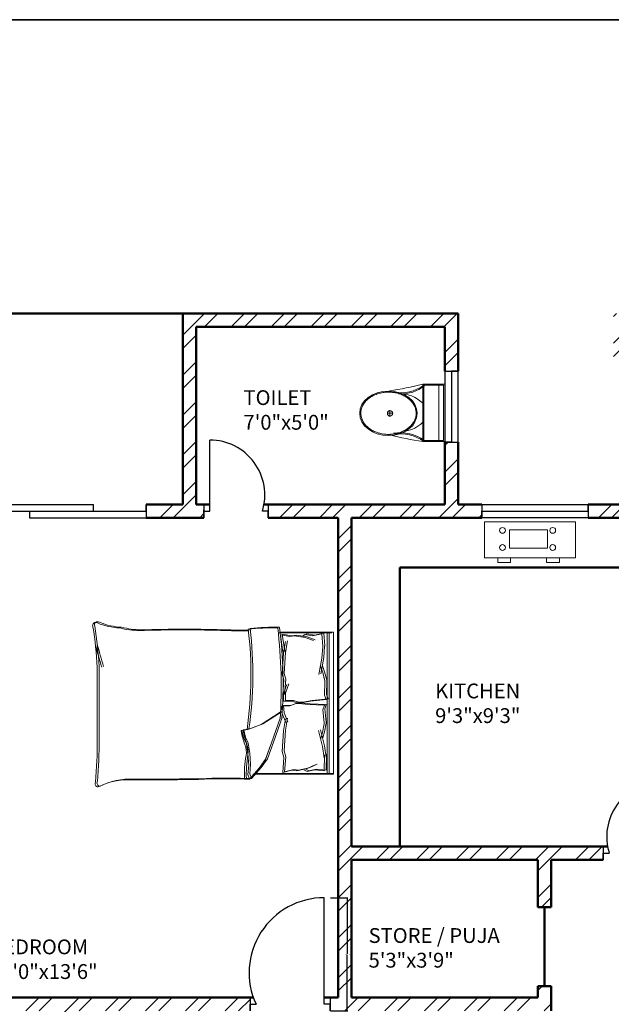
# Model space of a CAD drawing. Units: inches. Extents: x 963 to 2075, y 289 to 2657.
# Tile 80 of 98: x 1149 to 1349, y 2325 to 2657. Entities that reach past the tile are written whole.
import ezdxf

# ---------------------------------------------------------------- set-up
doc = ezdxf.new("R2010")
doc.units = ezdxf.units.IN
for name, color, linetype, lineweight in [('A-ANNO-DIMS', 2, 'Continuous', 18), ('A-ANNO-TTLB', 7, 'Continuous', 35), ('A-AREA-IDEN', 7, 'Continuous', 18), ('A-DOOR', 4, 'Continuous', 25), ('A-FLOR-FIXT', 9, 'Continuous', 18), ('A-FURN', 8, 'Continuous', 18), ('A-GLAZ', 3, 'Continuous', 25), ('A-WALL', 7, 'Continuous', 50), ('A-WALL-PATT', 8, 'Continuous', 13)]:
    doc.layers.add(name, color=color, linetype=linetype, lineweight=lineweight)
doc.styles.get("Standard").update_dxf_attribs({"font": 'arial.ttf'})
doc.dimstyles.get("Standard").update_dxf_attribs({"dimtxt": 0.18, "dimasz": 0.18, "dimexe": 0.18, "dimexo": 0.0625, "dimgap": 0.09, "dimtad": 0, "dimtih": 1, "dimtoh": 1, "dimdec": 4, "dimzin": 0, "dimdsep": 46, "dimtxsty": 'Standard', "dimcen": 0.09, "dimadec": 0, "dimazin": 0, "dimtfac": 1, "dimtdec": 4, "dimtofl": 0, "dimtmove": 0, "dimatfit": 3, "dimfxl": 1, "dimtolj": 1, "dimtzin": 0, "dimarcsym": 0})

# ---------------------------------------------------------------- blocks, each defined once
blk = doc.blocks.new('A$C31115884')
for p, q in [((283.1, 497.7), (223.4, 497.7)), ((257.5, 466.4), (257.5, 523.2)), ((0, 200), (0, 0)), ((520, 200), (0, 200)), ((10, 190), (10, 10)), ((510, 190), (10, 190)), ((510, 10), (510, 190)), ((520, 0), (520, 200)), ((510, 54.5), (0, 54.5)), ((10, 10), (510, 10)), ((0, 0), (520, 0))]:
    blk.add_line(p, q)
blk.add_circle((255.6, 496.4), 23.6)
for centre, radius, start, end in [((2777.7, -204.6), 2807, 165.4549, 171.71327), ((-294.5, 403.3), 364.7, 324.20913, 9.34987), ((-294.5, 403.3), 374.7, 324.20913, 9.34987), ((805.8, 403.3), 364.7, 170.65013, 215.79087), ((3237, 905), 2807, 188.28673, 194.5451), ((139.5, 406.2), 293.5, 315.84364, 2.65635), ((805.8, 403.3), 374.7, 179.20365, 215.79087), ((383.6, 406.2), 293.5, 190.27735, 224.15636)]:
    blk.add_arc(centre, radius, start, end)
blk.add_ellipse((256.2, 509.9), major_axis=(0, -260.7), ratio=0.772727)
blk.add_open_spline([(256.2, 259.2), (263.1, 259.2), (270, 259.7), (287.8, 262.3), (298.7, 265.1), (319.9, 273.1), (330.2, 278.4), (350.1, 291.1), (359.7, 298.7), (377.7, 315.9), (386.2, 325.5), (401.7, 346.6), (408.8, 358.1), (421.3, 382.5), (426.8, 395.5), (435.9, 422.4), (439.5, 436.4), (444.8, 465.1), (446.5, 479.7), (447.9, 509.2), (447.6, 524), (445, 553.3), (442.7, 567.8), (436.3, 596), (432.1, 609.7), (421.9, 636), (416, 648.6), (402.5, 672.1), (395, 683), (378.6, 703), (369.8, 712.1), (351.1, 728), (341.3, 734.8), (320.9, 746.2), (310.4, 750.7), (288.9, 757.3), (278, 759.4), (256, 761), (245, 760.6), (223.1, 757.2), (212.3, 754.3), (191.1, 746.1), (180.8, 740.7), (160.9, 727.8), (151.4, 720.1), (133.5, 702.7), (125.1, 693), (109.6, 671.7), (102.6, 660.2), (90.2, 635.7), (84.9, 622.7), (76, 595.6), (72.4, 581.6), (67.2, 552.9), (65.6, 538.2), (64.4, 508.8), (64.8, 494), (67.5, 464.7), (69.9, 450.2), (76.6, 422), (80.8, 408.3), (91.1, 382.2), (97.2, 369.7), (110.8, 346.3), (118.4, 335.4), (134.8, 315.6), (143.7, 306.7), (162.4, 290.9), (172.3, 284.2), (192.8, 273), (203.3, 268.6), (224.8, 262.2), (235.8, 260.2), (249.9, 259.3), (253, 259.2), (256.2, 259.2)], degree=3, knots=[0, 0, 0, 0, 0.110105, 0.110105, 0.285049, 0.285049, 0.459994, 0.459994, 0.634938, 0.634938, 0.809882, 0.809882, 0.984827, 0.984827, 1.159771, 1.159771, 1.334715, 1.334715, 1.50966, 1.50966, 1.684604, 1.684604, 1.859549, 1.859549, 2.034493, 2.034493, 2.209437, 2.209437, 2.384382, 2.384382, 2.559326, 2.559326, 2.73427, 2.73427, 2.909215, 2.909215, 3.084159, 3.084159, 3.259103, 3.259103, 3.434048, 3.434048, 3.608992, 3.608992, 3.783936, 3.783936, 3.958881, 3.958881, 4.133825, 4.133825, 4.30877, 4.30877, 4.483714, 4.483714, 4.658658, 4.658658, 4.833603, 4.833603, 5.008547, 5.008547, 5.183491, 5.183491, 5.358436, 5.358436, 5.53338, 5.53338, 5.708324, 5.708324, 5.883269, 5.883269, 6.058213, 6.058213, 6.233158, 6.233158, 6.283185, 6.283185, 6.283185, 6.283185])
blk = doc.blocks.new('BED-DOUBLE')
for p, q in [((1236.12, 2450.52), (1254.23, 2450.52)), ((1236.12, 2450.52), (1254.23, 2450.52)), ((1236.76, 2450.75), (1254.87, 2450.75)), ((1236.76, 2450.75), (1254.87, 2450.75)), ((1238.25, 2444.94), (1237.53, 2450.04)), ((1237.53, 2450.04), (1240.71, 2449.46)), ((1238.25, 2444.94), (1237.53, 2450.04)), ((1237.53, 2450.04), (1240.71, 2449.46)), ((1245.77, 2450.18), (1244.76, 2449.61)), ((1245.77, 2450.18), (1244.76, 2449.61)), ((1248.37, 2449.75), (1245.77, 2450.18)), ((1248.37, 2449.75), (1245.77, 2450.18)), ((1250.92, 2450.1), (1247.74, 2449.52)), ((1250.92, 2450.1), (1247.74, 2449.52)), ((1251.56, 2450.33), (1248.37, 2449.75)), ((1251.56, 2450.33), (1248.37, 2449.75)), ((1250.89, 2450.1), (1251.22, 2445.82)), ((1250.89, 2450.1), (1251.22, 2445.82)), ((1251.53, 2450.32), (1251.86, 2446.04)), ((1251.53, 2450.32), (1251.86, 2446.04)), ((1252.7, 2450.52), (1252.7, 2402.73)), ((1252.7, 2450.52), (1252.7, 2402.73)), ((1253.34, 2450.75), (1253.34, 2402.96)), ((1253.34, 2450.75), (1253.34, 2402.96)), ((1254.87, 2450.75), (1254.87, 2402.73)), ((1237.61, 2444.71), (1236.89, 2449.81)), ((1236.89, 2449.81), (1240.07, 2449.23)), ((1237.61, 2444.71), (1236.89, 2449.81)), ((1236.89, 2449.81), (1240.07, 2449.23)), ((1238.6, 2447.61), (1237.94, 2443.58)), ((1238.6, 2447.61), (1237.94, 2443.58)), ((1239.24, 2447.84), (1238.58, 2443.81)), ((1239.24, 2447.84), (1238.58, 2443.81)), ((1240.07, 2449.23), (1241.66, 2449.52)), ((1240.07, 2449.23), (1241.66, 2449.52)), ((1240.71, 2449.46), (1242.3, 2449.75)), ((1240.71, 2449.46), (1242.3, 2449.75)), ((1241.66, 2449.52), (1245.28, 2448.94)), ((1241.66, 2449.52), (1245.28, 2448.94)), ((1242.3, 2449.75), (1245.92, 2449.17)), ((1242.3, 2449.75), (1245.92, 2449.17)), ((1245.13, 2449.96), (1244.12, 2449.38)), ((1245.13, 2449.96), (1244.12, 2449.38)), ((1247.74, 2449.52), (1245.13, 2449.96)), ((1247.74, 2449.52), (1245.13, 2449.96)), ((1245.28, 2448.94), (1248.02, 2447.93)), ((1245.28, 2448.94), (1248.02, 2447.93)), ((1245.92, 2449.17), (1248.66, 2448.16)), ((1245.92, 2449.17), (1248.66, 2448.16)), ((1237.94, 2443.58), (1237.51, 2436.57)), ((1237.94, 2443.58), (1237.51, 2436.57)), ((1237.94, 2443.58), (1237.61, 2444.71)), ((1237.94, 2443.58), (1237.61, 2444.71)), ((1238.58, 2443.81), (1238.15, 2436.8)), ((1238.58, 2443.81), (1238.15, 2436.8)), ((1238.58, 2443.81), (1238.25, 2444.94)), ((1238.58, 2443.81), (1238.25, 2444.94)), ((1251.21, 2445.71), (1250.92, 2441.89)), ((1251.21, 2445.71), (1250.92, 2441.89)), ((1251.22, 2445.82), (1251.21, 2445.71)), ((1251.22, 2445.82), (1251.21, 2445.71)), ((1251.84, 2445.94), (1251.56, 2442.11)), ((1251.84, 2445.94), (1251.56, 2442.11)), ((1251.86, 2446.04), (1251.84, 2445.94)), ((1251.86, 2446.04), (1251.84, 2445.94)), ((1250.92, 2441.89), (1249.9, 2436.39)), ((1250.92, 2441.89), (1249.9, 2436.39)), ((1251.56, 2442.11), (1250.54, 2436.62)), ((1251.56, 2442.11), (1250.54, 2436.62)), ((1174.99, 2438.93), (1174.99, 2414.32)), ((1174.99, 2438.93), (1174.99, 2414.32)), ((1175.63, 2439.16), (1175.63, 2414.55)), ((1175.63, 2439.16), (1175.63, 2414.55)), ((1238.15, 2436.8), (1238.7, 2434.84)), ((1238.15, 2436.8), (1238.7, 2434.84)), ((1250.48, 2439.14), (1251.21, 2437.12)), ((1250.48, 2439.14), (1251.21, 2437.12)), ((1251.12, 2439.37), (1251.84, 2437.34)), ((1251.12, 2439.37), (1251.84, 2437.34)), ((1251.21, 2437.12), (1251.93, 2434.22)), ((1251.21, 2437.12), (1251.93, 2434.23)), ((1251.84, 2437.34), (1252.57, 2434.45)), ((1251.84, 2437.34), (1252.57, 2434.45)), ((1237.51, 2436.57), (1238.06, 2434.61)), ((1237.51, 2436.57), (1238.06, 2434.61)), ((1238.06, 2434.61), (1237.66, 2429.48)), ((1238.06, 2434.61), (1237.66, 2429.48)), ((1238.7, 2434.84), (1238.3, 2429.71)), ((1238.7, 2434.84), (1238.3, 2429.71)), ((1251.93, 2433.9), (1251.78, 2429.46)), ((1251.93, 2433.9), (1251.78, 2429.46)), ((1251.93, 2434.23), (1251.93, 2433.9)), ((1251.93, 2434.22), (1251.93, 2433.9)), ((1252.57, 2434.13), (1252.42, 2429.69)), ((1252.57, 2434.13), (1252.42, 2429.69)), ((1252.57, 2434.45), (1252.57, 2434.13)), ((1252.57, 2434.45), (1252.57, 2434.13)), ((1237.97, 2429.89), (1239.06, 2433.04)), ((1237.97, 2429.89), (1239.06, 2433.04)), ((1238.61, 2430.12), (1239.7, 2433.26)), ((1238.61, 2430.12), (1239.7, 2433.26)), ((1238.61, 2427.66), (1238.61, 2430.12)), ((1238.61, 2427.66), (1238.61, 2430.12)), ((1237.97, 2427.43), (1237.97, 2429.89)), ((1237.97, 2427.43), (1237.97, 2429.89)), ((1240.65, 2427.43), (1237.97, 2427.43)), ((1240.65, 2427.43), (1237.97, 2427.43)), ((1241.29, 2427.66), (1238.61, 2427.66)), ((1241.29, 2427.66), (1238.61, 2427.66)), ((1242.53, 2426.86), (1240.65, 2427.43)), ((1242.53, 2426.86), (1240.65, 2427.43)), ((1242.49, 2426.79), (1240.66, 2426.09)), ((1242.49, 2426.79), (1240.66, 2426.09)), ((1243.17, 2427.08), (1241.29, 2427.66)), ((1243.17, 2427.08), (1241.29, 2427.66)), ((1243.79, 2426.87), (1242.49, 2426.79)), ((1243.79, 2426.87), (1242.49, 2426.79)), ((1243.83, 2426.86), (1242.53, 2426.86)), ((1243.83, 2426.86), (1242.53, 2426.86)), ((1244.47, 2427.08), (1243.17, 2427.08)), ((1244.47, 2427.08), (1243.17, 2427.08)), ((1247, 2426.49), (1243.79, 2426.87)), ((1247, 2426.49), (1243.79, 2426.87)), ((1247.01, 2427.43), (1243.83, 2426.86)), ((1247.01, 2427.43), (1243.83, 2426.86)), ((1247.65, 2427.66), (1244.47, 2427.08)), ((1247.65, 2427.66), (1244.47, 2427.08)), ((1252.36, 2428.01), (1247.01, 2427.43)), ((1252.36, 2428.01), (1247.01, 2427.43)), ((1253, 2428.24), (1247.65, 2427.66)), ((1253, 2428.24), (1247.65, 2427.66)), ((1251.78, 2429.46), (1252.36, 2428.01)), ((1251.78, 2429.46), (1252.36, 2428.01)), ((1252.42, 2429.69), (1253, 2428.24)), ((1252.42, 2429.69), (1253, 2428.24)), ((1236.85, 2423.74), (1230.36, 2419.55)), ((1236.85, 2423.74), (1230.36, 2419.55)), ((1237.49, 2423.96), (1231, 2419.77)), ((1237.49, 2423.96), (1231, 2419.77)), ((1240.02, 2425.86), (1237.34, 2425.7)), ((1240.02, 2425.86), (1237.34, 2425.7)), ((1237.34, 2425.7), (1237.49, 2423.24)), ((1237.34, 2425.7), (1237.49, 2423.24)), ((1240.66, 2426.09), (1237.98, 2425.93)), ((1240.66, 2426.09), (1237.98, 2425.93)), ((1237.98, 2425.93), (1238.13, 2423.47)), ((1237.98, 2425.93), (1238.13, 2423.47)), ((1238.13, 2423.47), (1239.42, 2420.4)), ((1238.13, 2423.47), (1239.42, 2420.4)), ((1241.86, 2426.56), (1240.02, 2425.86)), ((1241.86, 2426.56), (1240.02, 2425.86)), ((1243.15, 2426.64), (1241.86, 2426.56)), ((1243.15, 2426.64), (1241.86, 2426.56)), ((1246.37, 2426.26), (1243.15, 2426.64)), ((1246.37, 2426.26), (1243.15, 2426.64)), ((1251.74, 2426.02), (1246.37, 2426.26)), ((1251.74, 2426.02), (1246.37, 2426.26)), ((1252.38, 2426.25), (1247, 2426.49)), ((1252.38, 2426.25), (1247, 2426.49)), ((1251.25, 2424.54), (1251.74, 2426.02)), ((1251.25, 2424.54), (1251.74, 2426.02)), ((1251.68, 2420.11), (1251.25, 2424.54)), ((1251.68, 2420.11), (1251.25, 2424.54)), ((1251.89, 2424.77), (1252.38, 2426.25)), ((1251.89, 2424.77), (1252.38, 2426.25)), ((1252.31, 2420.34), (1251.89, 2424.77)), ((1252.31, 2420.34), (1251.89, 2424.77)), ((1233.92, 2413.35), (1236.85, 2421.69)), ((1233.92, 2413.35), (1236.85, 2421.69)), ((1234.56, 2413.58), (1237.49, 2421.92)), ((1234.56, 2413.58), (1237.49, 2421.92)), ((1237.49, 2423.24), (1238.78, 2420.17)), ((1237.49, 2423.24), (1238.78, 2420.17)), ((1238.6, 2421.43), (1237.94, 2417.4)), ((1238.6, 2421.43), (1237.94, 2417.4)), ((1239.24, 2421.66), (1238.58, 2417.63)), ((1239.24, 2421.66), (1238.58, 2417.63)), ((1251.7, 2419.79), (1251.68, 2420.11)), ((1251.7, 2419.79), (1251.68, 2420.11)), ((1252.33, 2420.02), (1252.31, 2420.34)), ((1252.33, 2420.02), (1252.31, 2420.34)), ((1225.87, 2417.84), (1223.86, 2417.53)), ((1225.87, 2417.84), (1223.86, 2417.53)), ((1223.86, 2417.53), (1224.47, 2415.05)), ((1223.86, 2417.53), (1224.47, 2415.05)), ((1226.51, 2418.07), (1224.49, 2417.76)), ((1226.51, 2418.07), (1224.49, 2417.76)), ((1224.49, 2417.76), (1225.11, 2415.28)), ((1224.49, 2417.76), (1225.11, 2415.28)), ((1230.36, 2419.55), (1225.87, 2417.84)), ((1230.36, 2419.55), (1225.87, 2417.84)), ((1231, 2419.77), (1226.51, 2418.07)), ((1231, 2419.77), (1226.51, 2418.07)), ((1237.94, 2417.4), (1237.51, 2410.39)), ((1237.94, 2417.4), (1237.51, 2410.39)), ((1238.58, 2417.63), (1238.15, 2410.62)), ((1238.58, 2417.63), (1238.15, 2410.62)), ((1251.16, 2412.08), (1249.81, 2417.5)), ((1251.16, 2412.08), (1249.81, 2417.5)), ((1251.8, 2412.31), (1250.45, 2417.73)), ((1251.8, 2412.31), (1250.45, 2417.73)), ((1250.56, 2414.79), (1251.15, 2416.86)), ((1250.56, 2414.79), (1251.15, 2416.86)), ((1251.15, 2416.86), (1251.7, 2419.79)), ((1251.15, 2416.86), (1251.7, 2419.79)), ((1251.2, 2415.02), (1251.79, 2417.09)), ((1251.2, 2415.02), (1251.79, 2417.09)), ((1251.79, 2417.09), (1252.33, 2420.02)), ((1251.79, 2417.09), (1252.33, 2420.02)), ((1224.47, 2415.05), (1225.4, 2413.04)), ((1224.47, 2415.05), (1225.4, 2413.04)), ((1225.11, 2415.28), (1226.04, 2413.27)), ((1225.11, 2415.28), (1226.04, 2413.27)), ((1232.54, 2408), (1234.56, 2413.58)), ((1232.54, 2408), (1234.56, 2413.58)), ((1225.4, 2413.04), (1225.87, 2409.63)), ((1225.4, 2413.04), (1225.87, 2409.63)), ((1226.04, 2413.27), (1226.51, 2409.86)), ((1226.04, 2413.27), (1226.51, 2409.86)), ((1231.9, 2407.77), (1233.92, 2413.35)), ((1231.9, 2407.78), (1233.92, 2413.35)), ((1237.51, 2410.39), (1238.06, 2408.43)), ((1237.51, 2410.39), (1238.06, 2408.43)), ((1238.15, 2410.62), (1238.7, 2408.66)), ((1238.15, 2410.62), (1238.7, 2408.66)), ((1251.69, 2408.28), (1251.16, 2412.08)), ((1251.69, 2408.28), (1251.16, 2412.08)), ((1252.33, 2408.51), (1251.8, 2412.31)), ((1252.33, 2408.51), (1251.8, 2412.31)), ((1225.87, 2409.63), (1226.18, 2405.76)), ((1225.87, 2409.63), (1226.18, 2405.76)), ((1226.51, 2409.86), (1226.82, 2405.99)), ((1226.51, 2409.86), (1226.82, 2405.99)), ((1229.74, 2404.83), (1231.9, 2407.78)), ((1229.74, 2404.83), (1231.9, 2407.77)), ((1230.38, 2405.06), (1232.54, 2408)), ((1230.38, 2405.06), (1232.54, 2408)), ((1238.06, 2408.43), (1237.66, 2403.3)), ((1238.06, 2408.43), (1237.66, 2403.3)), ((1238.7, 2408.66), (1238.3, 2403.52)), ((1238.7, 2408.66), (1238.3, 2403.52)), ((1251.68, 2403.88), (1251.77, 2409.29)), ((1251.68, 2403.88), (1251.77, 2409.28)), ((1251.77, 2409.29), (1251.69, 2408.28)), ((1251.77, 2409.28), (1251.69, 2408.28)), ((1252.31, 2404.11), (1252.41, 2409.51)), ((1252.31, 2404.11), (1252.41, 2409.51)), ((1252.41, 2409.51), (1252.33, 2408.51)), ((1252.41, 2409.51), (1252.33, 2408.51)), ((1226.18, 2405.76), (1225.87, 2402.66)), ((1226.18, 2405.76), (1225.87, 2402.66)), ((1226.49, 2401.13), (1229.74, 2404.83)), ((1226.49, 2401.13), (1229.74, 2404.83)), ((1226.82, 2405.99), (1226.51, 2402.89)), ((1226.82, 2405.99), (1226.51, 2402.89)), ((1227.13, 2401.36), (1230.38, 2405.06)), ((1227.13, 2401.36), (1230.38, 2405.06)), ((1237.66, 2403.3), (1240.8, 2404.07)), ((1237.66, 2403.3), (1240.8, 2404.07)), ((1238.3, 2403.52), (1241.44, 2404.3)), ((1238.3, 2403.52), (1241.44, 2404.3)), ((1240.8, 2404.07), (1242.4, 2403.88)), ((1240.8, 2404.07), (1242.4, 2403.88)), ((1241.44, 2404.3), (1243.04, 2404.11)), ((1241.44, 2404.3), (1243.04, 2404.11)), ((1242.4, 2403.88), (1245.98, 2404.69)), ((1242.4, 2403.88), (1245.98, 2404.69)), ((1243.04, 2404.11), (1246.61, 2404.91)), ((1243.04, 2404.11), (1246.61, 2404.91)), ((1245.89, 2403.67), (1244.85, 2404.18)), ((1245.89, 2403.67), (1244.85, 2404.18)), ((1246.53, 2403.89), (1245.49, 2404.41)), ((1246.53, 2403.89), (1245.49, 2404.41)), ((1248.46, 2404.26), (1245.89, 2403.67)), ((1248.46, 2404.26), (1245.89, 2403.67)), ((1245.98, 2404.69), (1248.65, 2405.87)), ((1245.98, 2404.69), (1248.65, 2405.87)), ((1249.1, 2404.49), (1246.53, 2403.89)), ((1249.1, 2404.49), (1246.53, 2403.89)), ((1246.61, 2404.91), (1249.29, 2406.1)), ((1246.61, 2404.91), (1249.29, 2406.09)), ((1251.68, 2403.88), (1248.46, 2404.26)), ((1251.68, 2403.88), (1248.46, 2404.26)), ((1252.31, 2404.11), (1249.1, 2404.49)), ((1252.31, 2404.11), (1249.1, 2404.49)), ((1224.74, 2401.05), (1226.49, 2401.13, 3.87)), ((1224.74, 2401.05), (1226.49, 2401.13, 3.87)), ((1225.38, 2401.28), (1227.13, 2401.36, 3.87)), ((1225.38, 2401.28), (1227.13, 2401.36, 3.87)), ((1225.87, 2402.66), (1226.49, 2401.13)), ((1225.87, 2402.66), (1226.49, 2401.13)), ((1226.51, 2402.89), (1227.13, 2401.36)), ((1226.51, 2402.89), (1227.13, 2401.36)), ((1254.23, 2402.73), (1227.62, 2402.73)), ((1254.23, 2402.73), (1227.62, 2402.73)), ((1254.87, 2402.96), (1228.26, 2402.96)), ((1254.87, 2402.96), (1228.26, 2402.96)), ((1254.87, 2402.73), (1254.23, 2402.73))]:
    blk.add_line(p, q)
for centre, radius, start, end in [((1174.51, 2452.91), 1.09, 56.1736, 203.4781), ((1174.51, 2452.91), 1.09, 56.1736, 203.4781), ((1175.15, 2453.14), 1.09, 56.1736, 203.4781), ((1175.15, 2453.14), 1.09, 56.1736, 203.4781), ((1183.96, 2475.65), 23.56, 247.9751, 266.652), ((1183.96, 2475.65), 23.56, 247.9751, 266.652), ((1184.6, 2475.88), 23.56, 247.9751, 266.652), ((1184.6, 2475.88), 23.56, 247.9751, 266.652), ((1053.4, 2432.57), 121.76, 2.9958, 9.4091), ((1053.4, 2432.57), 121.76, 2.9958, 9.4091), ((1054.03, 2432.8), 121.76, 2.9958, 9.4091), ((1054.03, 2432.8), 121.76, 2.9958, 9.4091), ((1189.72, 2480.89), 29.63, 256.0648, 268.9113), ((1189.72, 2480.89), 29.63, 256.0648, 268.9113), ((1190.36, 2481.12), 29.63, 256.0648, 268.9113), ((1190.36, 2481.12), 29.63, 256.0648, 268.9113), ((1203.62, 1969.17), 482.31, 88.2277, 91.7185), ((1203.62, 1969.17), 482.31, 88.2277, 91.7185), ((1204.26, 1969.4), 482.31, 88.2277, 91.7185), ((1204.26, 1969.4), 482.31, 88.2277, 91.7185), ((1223.06, 2621.3), 170.11, 268.4762, 271.0082), ((1223.06, 2621.3), 170.11, 268.4762, 271.0082), ((1223.7, 2621.53), 170.11, 268.4762, 271.0082), ((1223.7, 2621.53), 170.11, 268.4762, 271.0082), ((1097.92, 2436.24), 129.02, 351.7845, 6.9006), ((1097.92, 2436.24), 129.02, 351.7845, 6.9006), ((1234.14, 2368.83), 83.31, 88.7218, 95.604), ((1234.14, 2368.83), 83.31, 88.7218, 95.604), ((1098.56, 2436.47), 129.02, 351.7845, 6.9006), ((1098.56, 2436.47), 129.02, 351.7845, 6.9006), ((1234.78, 2369.06), 83.31, 88.7218, 95.604), ((1234.78, 2369.06), 83.31, 88.7218, 95.604), ((1072.18, 2432.64), 164.97, 356.0865, 6.7821), ((1072.18, 2432.64), 164.97, 356.0865, 6.7821), ((1072.82, 2432.86), 164.97, 356.0865, 6.7821), ((1072.82, 2432.86), 164.97, 356.0865, 6.7821), ((1278.58, 2471.44), 106.46, 193.3832, 197.7053), ((1278.58, 2471.44), 106.46, 193.3832, 197.7053), ((1277.94, 2471.22), 106.46, 193.3832, 197.7053), ((1277.94, 2471.22), 106.46, 193.3832, 197.7053), ((1223.79, 2417.36), 0.185, 70.2464, 181.1377), ((1223.79, 2417.36), 0.185, 70.2464, 181.1377), ((1252.75, 2422.84), 29.65, 190.6617, 199.8806), ((1252.75, 2422.84), 29.65, 190.6617, 199.8806), ((1224.43, 2417.59), 0.185, 70.2464, 181.1377), ((1224.43, 2417.59), 0.185, 70.2464, 181.1377), ((1253.39, 2423.07), 29.65, 190.6617, 199.8806), ((1253.39, 2423.07), 29.65, 190.6617, 199.8806), ((1041.96, 2412.84), 133.04, 354.4998, 0.6351), ((1041.96, 2412.84), 133.04, 354.4998, 0.6351), ((1042.6, 2413.07), 133.04, 354.4998, 0.6351), ((1042.6, 2413.07), 133.04, 354.4998, 0.6351), ((1219.17, 2410.25), 6.22, 348.6608, 23.7384), ((1219.17, 2410.25), 6.22, 348.6608, 23.7384), ((1219.81, 2410.48), 6.22, 348.6608, 23.7384), ((1219.81, 2410.48), 6.22, 348.6608, 23.7384), ((1260.89, 2402.67), 36.18, 169.8763, 182.5657), ((1260.89, 2402.67), 36.18, 169.8763, 182.5657), ((1261.53, 2402.9), 36.18, 169.8763, 182.5657), ((1261.53, 2402.9), 36.18, 169.8763, 182.5657), ((1176, 2399.81), 1.1, 152.6588, 266.02), ((1176, 2399.81), 1.1, 152.6588, 266.02), ((1185.57, 2377.84), 23.07, 87.4714, 116.4681), ((1185.57, 2377.84), 23.07, 87.4714, 116.4681), ((1186.21, 2378.07), 23.07, 87.4714, 116.4681), ((1186.21, 2378.07), 23.07, 87.4714, 116.4681), ((1186.41, 6962.74), 4561.86, 270.00217, 270.28689), ((1186.41, 6962.74), 4561.86, 270.00217, 270.28689), ((1187.05, 6962.97), 4561.86, 270.00217, 270.28689), ((1187.05, 6962.97), 4561.86, 270.00217, 270.28689), ((1217.92, 2271.73), 129.5, 86.9791, 93.8365), ((1217.92, 2271.73), 129.5, 86.9791, 93.8365), ((1218.56, 2271.96), 129.5, 86.9791, 93.8365), ((1218.56, 2271.96), 129.5, 86.9791, 93.8365), ((1175.36, 2399.58), 1.1, 152.6588, 266.02), ((1175.36, 2399.58), 1.1, 152.6588, 266.02)]:
    blk.add_arc(centre, radius, start, end)
blk = doc.blocks.new('KITCHEN-SINK')
for points in [[(-0.1, 14), (30.59, 14), (30.59, 1.84), (-0.1, 1.84)], [(8.33, 11.28), (21.1, 11.28), (21.1, 5.02), (8.33, 5.02)], [(4.31, 1.84), (8.69, 1.84), (8.69, 0.24), (4.31, 0.24)], [(20.79, 1.84), (25.17, 1.84), (25.17, 0.24), (20.79, 0.24)]]:
    blk.add_lwpolyline(points, close=True)
for centre in [(5.94, 11.08), (22.9, 11.08), (5.94, 5.28), (22.9, 5.28)]:
    blk.add_circle(centre, 0.978)
blk = doc.blocks.new('DOOR-1')
for p, q in [((25.38, 2.25), (25.38, 38.25)), ((0.32, 4.5), (0.32, 0)), ((27.38, 4.5), (27.38, 0)), ((0.32, 0), (0.32, 2.25)), ((0.32, 2.25), (2.32, 2.25)), ((27.38, 2.25), (25.38, 2.25)), ((27.38, 0), (27.38, 2.25))]:
    blk.add_line(p, q)
blk.add_arc((25.38, 12.86), 25.39, 90, 204.7158)
blk = doc.blocks.new('*D30')
at = {"layer": 'A-ANNO-DIMS', "color": 0, "lineweight": -2, "transparency": 16777216}
for p, q in [((1253.78, 2361.07), (1259.63, 2361.07)), ((1259.45, 2360.89), (1259.45, 2342.13)), ((1259.45, 2323), (1259.45, 2341.76)), ((1253.78, 2322.82), (1259.63, 2322.82))]:
    blk.add_line(p, q, dxfattribs=at)
at = {"layer": 'A-ANNO-DIMS', "color": 0, "transparency": 16777216}
for points in [[(1259.42, 2360.89), (1259.48, 2360.89), (1259.45, 2361.07)], [(1259.42, 2323), (1259.48, 2323), (1259.45, 2322.82)]]:
    blk.add_solid(points, dxfattribs=at)
at = {"layer": 'Defpoints', "color": 0, "transparency": 16777216}
for p in [(1253.71, 2361.07), (1259.45, 2361.07), (1253.71, 2322.82)]:
    blk.add_point(p, dxfattribs=at)
at = {"layer": 'A-ANNO-DIMS', "color": 0, "transparency": 16777216, "insert": (1259.45, 2341.94), "char_height": 0.18, "attachment_point": 5}
blk.add_mtext('\\A1;DOOR D1 38 TYP.', dxfattribs=at)

msp = doc.modelspace()

# ---------------------------------------------------------------- hatches: boundary and pattern name
at = {"layer": 'A-WALL-PATT'}
h = msp.add_hatch(dxfattribs=at)
h.set_pattern_fill('ANSI32', color=256)
h.paths.add_polyline_path([(1296.92, 2558.32), (1203.92, 2558.32), (1203.92, 2493.82), (1191.53, 2493.82), (1191.53, 2489.32), (1211.06, 2489.32), (1211.06, 2492.02), (1211.06, 2493.82), (1208.42, 2493.82), (1208.42, 2553.82), (1292.42, 2553.82), (1292.42, 2538.86), (1296.92, 2538.86)])
h.paths.add_polyline_path([(1442.42, 2558.32), (1349.42, 2558.32), (1349.42, 2538.94), (1353.92, 2538.94), (1353.92, 2553.82), (1437.92, 2553.82), (1437.92, 2493.82), (1434.54, 2493.82), (1434.54, 2489.32), (1448.31, 2489.32), (1448.31, 2491.57), (1448.31, 2493.82), (1442.42, 2493.82)])
h.paths.add_polyline_path([(1415.55, 2491.57), (1415.55, 2493.82), (1340.94, 2493.82), (1340.94, 2489.32), (1371.92, 2489.32), (1371.92, 2378.32), (1367.6, 2378.32), (1367.6, 2373.82), (1371.92, 2373.82), (1371.92, 2355.19), (1376.42, 2355.19), (1376.42, 2489.32), (1415.55, 2489.32)])
h.paths.add_polyline_path([(1304.94, 2491.57), (1304.94, 2493.82), (1296.92, 2493.82), (1296.92, 2514.86), (1292.42, 2514.86), (1292.42, 2493.82), (1232.81, 2493.82), (1232.81, 2489.32), (1256.42, 2489.32), (1256.42, 2327.32), (1253.71, 2327.32), (1253.71, 2322.82), (1328.42, 2322.82), (1328.42, 2331.15), (1323.92, 2331.15), (1323.92, 2327.32), (1260.92, 2327.32), (1260.92, 2373.82), (1323.92, 2373.82), (1323.92, 2357.81), (1328.42, 2357.81), (1328.42, 2373.82), (1346.01, 2373.82), (1346.01, 2376.07), (1346.01, 2378.32), (1260.92, 2378.32), (1260.92, 2489.32), (1304.94, 2489.32)])
h.paths.add_polyline_path([(1226.65, 2327.32), (1124.42, 2327.32), (1124.42, 2347.45), (1119.92, 2347.45), (1119.92, 2322.82), (1163.42, 2322.82), (1163.42, 2305.43), (1165.67, 2305.43), (1167.92, 2305.43), (1167.92, 2322.82), (1226.65, 2322.82), (1226.65, 2325.07)])
h.paths.add_polyline_path([(1095.92, 2489.32), (1124.42, 2489.32), (1131.53, 2489.32), (1131.53, 2491.57), (1131.53, 2493.82), (1119.92, 2493.82), (1091.42, 2493.82), (1091.42, 2417.32), (1095.92, 2417.32), (1119.92, 2417.32), (1119.92, 2407.45), (1124.42, 2407.45), (1124.42, 2421.82), (1095.92, 2421.82)])
h.paths.add_polyline_path([(1512.92, 2558.32), (1508.42, 2558.32), (1508.42, 2493.82), (1503.4, 2493.82), (1503.4, 2489.32), (1508.42, 2489.32), (1508.42, 2327.32), (1376.42, 2327.32), (1376.42, 2330.27), (1371.92, 2330.27), (1371.92, 2298.74), (1376.42, 2298.74), (1376.42, 2322.82), (1508.42, 2322.82), (1508.42, 2165.32), (1504.26, 2165.32), (1504.26, 2160.82), (1508.42, 2160.82), (1508.42, 2108.32), (1512.92, 2108.32), (1512.92, 2160.82), (1516.18, 2160.82), (1516.18, 2163.07), (1516.18, 2165.32), (1512.92, 2165.32), (1512.92, 2322.82), (1644.92, 2322.82), (1644.92, 2298.74), (1649.42, 2298.74), (1649.42, 2322.82), (1649.42, 2330.94), (1647.17, 2330.94), (1644.92, 2330.94), (1644.92, 2327.32), (1512.92, 2327.32), (1512.92, 2489.32), (1516.76, 2489.32), (1516.76, 2491.57), (1516.76, 2493.82), (1512.92, 2493.82)])
h.paths.add_polyline_path([(1671.92, 2558.32), (1578.92, 2558.32), (1578.92, 2493.82), (1573.53, 2493.82), (1573.53, 2489.32), (1586.54, 2489.32), (1586.54, 2491.57), (1586.54, 2493.82), (1583.42, 2493.82), (1583.42, 2553.82), (1667.42, 2553.82), (1667.42, 2541.11), (1671.92, 2541.11)])
h.paths.add_polyline_path([(1681.26, 2493.82), (1671.92, 2493.82), (1671.92, 2517.11), (1667.42, 2517.11), (1667.42, 2493.82), (1610.22, 2493.82), (1610.22, 2489.32), (1644.92, 2489.32), (1644.92, 2357.87), (1649.42, 2357.87), (1649.42, 2373.82), (1652.2, 2373.82), (1652.2, 2375.83), (1652.2, 2378.32), (1649.42, 2378.32), (1649.42, 2489.32), (1681.26, 2489.32), (1681.26, 2491.57)])
h.paths.add_polyline_path([(1821.92, 2558.32), (1728.92, 2558.32), (1728.92, 2541), (1733.42, 2541), (1733.42, 2553.82), (1817.42, 2553.82), (1817.42, 2493.82), (1813.51, 2493.82), (1813.51, 2489.32), (1830.08, 2489.32), (1830.08, 2491.57), (1830.08, 2493.82), (1821.92, 2493.82)])
h.paths.add_polyline_path([(1794.24, 2493.82), (1717.26, 2493.82), (1717.26, 2489.32), (1760.42, 2489.32), (1760.42, 2378.32), (1674.4, 2378.32), (1674.4, 2373.82), (1692.92, 2373.82), (1692.92, 2356.95), (1697.42, 2356.95), (1697.42, 2373.82), (1760.42, 2373.82), (1760.42, 2327.32), (1697.42, 2327.32), (1697.42, 2333.34), (1692.92, 2333.34), (1692.92, 2322.82), (1768.04, 2322.82), (1768.04, 2325.07), (1768.04, 2327.32), (1764.92, 2327.32), (1764.92, 2489.32), (1794.24, 2489.32)])
h.paths.add_polyline_path([(1733.42, 2517), (1728.92, 2517), (1728.92, 2493.82), (1733.42, 2493.82)], flags=17)
h.paths.add_polyline_path([(1929.92, 2493.82), (1890.08, 2493.82), (1890.08, 2489.32), (1896.92, 2489.32), (1925.42, 2489.32), (1925.42, 2421.82), (1896.92, 2421.82), (1896.92, 2408.32), (1901.42, 2408.32), (1901.42, 2417.32), (1925.42, 2417.32), (1929.92, 2417.32)])
h.paths.add_polyline_path([(1901.42, 2348.32), (1896.92, 2348.32), (1896.92, 2327.32), (1800.42, 2327.32), (1800.42, 2322.82), (1853.42, 2322.82), (1853.42, 2309.45), (1857.92, 2309.45), (1857.92, 2322.82), (1901.42, 2322.82)])
h.paths.add_polyline_path([(1857.92, 2249.45), (1853.42, 2249.45), (1853.42, 2214.82), (1686.31, 2214.82), (1686.31, 2210.32), (1853.42, 2210.32), (1853.42, 2202.13), (1857.92, 2202.13), (1857.92, 2210.32)])
h.paths.add_polyline_path([(1857.92, 2142.13), (1853.42, 2142.13), (1853.42, 2115.42), (1841.42, 2115.42), (1841.42, 2088.53), (1841.42, 2046.95), (1845.92, 2046.95), (1845.92, 2110.92), (1905.92, 2110.92), (1905.92, 2092.52), (1910.42, 2092.52), (1910.42, 2115.42), (1857.92, 2115.42)])
h.paths.add_polyline_path([(1532.44, 1482.34), (1573.46, 1482.34), (1573.46, 1501), (1532.44, 1501)], flags=9)
h.paths.add_polyline_path([(1438.66, 1486.3), (1479.68, 1486.3), (1479.68, 1504.96), (1438.66, 1504.96)], flags=9)
h.paths.add_polyline_path([(1411.22, 1365.31), (1659.14, 1365.31), (1659.14, 1402.4), (1411.22, 1402.4)], flags=9)
h.paths.add_polyline_path([(1185.67, 2296.3), (1248.16, 2296.3), (1248.16, 2314.95), (1185.67, 2314.95)], flags=9)
h.paths.add_polyline_path([(1177.31, 2187.35), (1216.15, 2187.35), (1216.15, 2206.01), (1177.31, 2206.01)], flags=9)
h.paths.add_polyline_path([(1295.1, 1602.08), (1328.26, 1602.08), (1328.26, 1620.74), (1295.1, 1620.74)], flags=9)
h.paths.add_polyline_path([(1525.13, 2005.99), (1558.39, 2005.99), (1558.39, 2024.65), (1525.13, 2024.65)], flags=9)
h.paths.add_polyline_path([(1459.61, 1977.13), (1472.19, 1977.13), (1472.19, 1987.43), (1459.61, 1987.43)], flags=9)
h.paths.add_polyline_path([(1467.81, 2053.68), (1480.02, 2053.68), (1480.02, 2063.98), (1467.81, 2063.98)], flags=9)
h.paths.add_polyline_path([(1555.18, 2119.02), (1584.56, 2119.02), (1584.56, 2137.68), (1555.18, 2137.68)], flags=25)
h.paths.add_polyline_path([(1405.39, 2115.29), (1444.48, 2115.29), (1444.48, 2133.95), (1405.39, 2133.95)], flags=25)
h.paths.add_polyline_path([(1698.48, 2004.26), (1727.69, 2004.26), (1727.69, 2022.92), (1698.48, 2022.92)], flags=9)
h.paths.add_polyline_path([(1612.16, 1972.86), (1629.02, 1972.86), (1629.02, 1983.16), (1612.16, 1983.16)], flags=9)
h.paths.add_polyline_path([(1608.29, 2060.04), (1625.15, 2060.04), (1625.15, 2070.34), (1608.29, 2070.34)], flags=9)
h.paths.add_polyline_path([(1527.95, 1684.4), (1566.79, 1684.4), (1566.79, 1703.06), (1527.95, 1703.06)], flags=9)
h.paths.add_polyline_path([(1422.79, 1683.59), (1461.63, 1683.59), (1461.63, 1702.25), (1422.79, 1702.25)], flags=9)
h.paths.add_polyline_path([(1531.26, 1732.46), (1574.01, 1732.46), (1574.01, 1751.12), (1531.26, 1751.12)], flags=9)
h.paths.add_polyline_path([(1402.87, 1732.85), (1439.8, 1732.85), (1439.8, 1751.5), (1402.87, 1751.5)], flags=9)
h.paths.add_polyline_path([(1243.12, 1923.13), (1281.96, 1923.13), (1281.96, 1941.79), (1243.12, 1941.79)], flags=9)
h.paths.add_polyline_path([(1181.75, 1792.27), (1244.24, 1792.27), (1244.24, 1810.93), (1181.75, 1810.93)], flags=9)
h.paths.add_polyline_path([(1265.82, 1670.3), (1316.07, 1670.3), (1316.07, 1688.96), (1265.82, 1688.96)], flags=9)
h.paths.add_polyline_path([(1140.26, 1676.05), (1179.1, 1676.05), (1179.1, 1694.71), (1140.26, 1694.71)], flags=9)
h.paths.add_polyline_path([(1107.49, 1490.89), (1143.37, 1490.89), (1143.37, 1509.55), (1107.49, 1509.55)], flags=9)
h.paths.add_polyline_path([(1217.58, 1483.9), (1246.74, 1483.9), (1246.74, 1502.56), (1217.58, 1502.56)], flags=9)
h.paths.add_polyline_path([(1389.21, 1486.92), (1418.37, 1486.92), (1418.37, 1505.58), (1389.21, 1505.58)], flags=9)
h.paths.add_polyline_path([(1672.21, 1602.08), (1705.37, 1602.08), (1705.37, 1620.74), (1672.21, 1620.74)], flags=9)
h.paths.add_polyline_path([(1752.08, 1522.64), (1781.24, 1522.64), (1781.24, 1541.3), (1752.08, 1541.3)], flags=9)
h.paths.add_polyline_path([(1848.27, 1491.26), (1884.16, 1491.26), (1884.16, 1509.92), (1848.27, 1509.92)], flags=9)
h.paths.add_polyline_path([(1822.47, 1685.62), (1861.31, 1685.62), (1861.31, 1704.28), (1822.47, 1704.28)], flags=9)
h.paths.add_polyline_path([(1713.19, 1672.23), (1763.44, 1672.23), (1763.44, 1690.89), (1713.19, 1690.89)], flags=9)
h.paths.add_polyline_path([(1736.62, 1790.58), (1799.11, 1790.58), (1799.11, 1809.24), (1736.62, 1809.24)], flags=9)
h.paths.add_polyline_path([(1691.49, 1916.36), (1730.33, 1916.36), (1730.33, 1935.01), (1691.49, 1935.01)], flags=9)
h.paths.add_polyline_path([(1764.87, 1973.92), (1794.31, 1973.92), (1794.31, 1992.58), (1764.87, 1992.58)], flags=9)
h.paths.add_polyline_path([(1767.85, 2034.02), (1797.29, 2034.02), (1797.29, 2052.67), (1767.85, 2052.67)], flags=9)
h.paths.add_polyline_path([(1851.59, 2060.33), (1880.75, 2060.33), (1880.75, 2078.99), (1851.59, 2078.99)], flags=25)
h.paths.add_polyline_path([(1688.49, 2086.87), (1727.33, 2086.87), (1727.33, 2105.53), (1688.49, 2105.53)], flags=9)
h.paths.add_polyline_path([(1537.74, 2293.58), (1580.49, 2293.58), (1580.49, 2312.24), (1537.74, 2312.24)], flags=25)
h.paths.add_polyline_path([(1425.59, 2296.11), (1468.34, 2296.11), (1468.34, 2314.77), (1425.59, 2314.77)], flags=25)
h.paths.add_polyline_path([(1278.52, 2004.18), (1307.72, 2004.18), (1307.72, 2022.84), (1278.52, 2022.84)], flags=9)
h.paths.add_polyline_path([(1193.28, 1973.63), (1222.72, 1973.63), (1222.72, 1992.29), (1193.28, 1992.29)], flags=9)
h.paths.add_polyline_path([(1192.41, 2040.58), (1221.84, 2040.58), (1221.84, 2059.23), (1192.41, 2059.23)], flags=9)
h.paths.add_polyline_path([(1130.6, 1951.39), (1159.76, 1951.39), (1159.76, 1970.05), (1130.6, 1970.05)], flags=9)
h.paths.add_polyline_path([(1132.83, 2052.49), (1161.98, 2052.49), (1161.98, 2071.15), (1132.83, 2071.15)], flags=9)
h.paths.add_polyline_path([(1265.13, 2334.62), (1315.38, 2334.62), (1315.38, 2353.28), (1265.13, 2353.28)], flags=25)
h.paths.add_polyline_path([(1136.74, 2330.79), (1175.58, 2330.79), (1175.58, 2349.44), (1136.74, 2349.44)], flags=9)
h.paths.add_polyline_path([(1287.42, 2417.2), (1320.58, 2417.2), (1320.58, 2435.86), (1287.42, 2435.86)], flags=25)
h.paths.add_polyline_path([(1430.99, 2329.16), (1469.83, 2329.16), (1469.83, 2347.82), (1430.99, 2347.82)], flags=25)
h.paths.add_polyline_path([(1525.42, 2329.21), (1564.26, 2329.21), (1564.26, 2347.87), (1525.42, 2347.87)], flags=25)
h.paths.add_polyline_path([(1684.52, 2382.8), (1717.68, 2382.8), (1717.68, 2401.46), (1684.52, 2401.46)], flags=25)
h.paths.add_polyline_path([(1704.81, 2340.29), (1755.05, 2340.29), (1755.05, 2358.95), (1704.81, 2358.95)], flags=25)
h.paths.add_polyline_path([(1694.11, 2287.76), (1756.6, 2287.76), (1756.6, 2306.41), (1694.11, 2306.41)], flags=9)
h.paths.add_polyline_path([(1815.78, 2329.86), (1854.62, 2329.86), (1854.62, 2348.52), (1815.78, 2348.52)], flags=9)
h.paths.add_polyline_path([(1842.87, 2514.26), (1878.76, 2514.26), (1878.76, 2532.91), (1842.87, 2532.91)], flags=9)
h.paths.add_polyline_path([(1769.51, 2531.45), (1798.67, 2531.45), (1798.67, 2550.1), (1769.51, 2550.1)], flags=25)
h.paths.add_polyline_path([(1594.77, 2518.47), (1623.93, 2518.47), (1623.93, 2537.13), (1594.77, 2537.13)], flags=25)
h.paths.add_polyline_path([(1520.72, 2516.18), (1556.61, 2516.18), (1556.61, 2534.84), (1520.72, 2534.84)], flags=25)
h.paths.add_polyline_path([(1464.46, 2516.69), (1500.34, 2516.69), (1500.34, 2535.35), (1464.46, 2535.35)], flags=25)
h.paths.add_polyline_path([(1365.7, 2528.97), (1394.85, 2528.97), (1394.85, 2547.63), (1365.7, 2547.63)], flags=25)
h.paths.add_polyline_path([(1222.84, 2516.23), (1252, 2516.23), (1252, 2534.89), (1222.84, 2534.89)], flags=25)
h.paths.add_polyline_path([(1104.55, 2509.6), (1140.43, 2509.6), (1140.43, 2528.26), (1104.55, 2528.26)], flags=9)
h = msp.add_hatch(dxfattribs=at)
h.set_pattern_fill('ANSI32', color=256)
h.paths.add_polyline_path([(1335.97, 2212.57), (1335.97, 2214.82), (1167.92, 2214.82), (1167.92, 2245.43), (1163.42, 2245.43), (1163.42, 2210.32), (1163.42, 2194.81), (1167.92, 2194.81), (1167.92, 2210.32), (1335.97, 2210.32)])
h.paths.add_polyline_path([(1532.44, 1482.34), (1573.46, 1482.34), (1573.46, 1501), (1532.44, 1501)], flags=9)
h.paths.add_polyline_path([(1438.66, 1486.3), (1479.68, 1486.3), (1479.68, 1504.96), (1438.66, 1504.96)], flags=9)
h.paths.add_polyline_path([(1411.22, 1365.31), (1659.14, 1365.31), (1659.14, 1402.4), (1411.22, 1402.4)], flags=9)
h.paths.add_polyline_path([(1185.67, 2296.3), (1248.16, 2296.3), (1248.16, 2314.95), (1185.67, 2314.95)], flags=9)
h.paths.add_polyline_path([(1177.31, 2187.35), (1216.15, 2187.35), (1216.15, 2206.01), (1177.31, 2206.01)], flags=9)
h.paths.add_polyline_path([(1295.1, 1602.08), (1328.26, 1602.08), (1328.26, 1620.74), (1295.1, 1620.74)], flags=9)
h.paths.add_polyline_path([(1525.13, 2005.99), (1558.39, 2005.99), (1558.39, 2024.65), (1525.13, 2024.65)], flags=9)
h.paths.add_polyline_path([(1459.61, 1977.13), (1472.19, 1977.13), (1472.19, 1987.43), (1459.61, 1987.43)], flags=9)
h.paths.add_polyline_path([(1467.81, 2053.68), (1480.02, 2053.68), (1480.02, 2063.98), (1467.81, 2063.98)], flags=9)
h.paths.add_polyline_path([(1555.18, 2119.02), (1584.56, 2119.02), (1584.56, 2137.68), (1555.18, 2137.68)], flags=9)
h.paths.add_polyline_path([(1405.39, 2115.29), (1444.48, 2115.29), (1444.48, 2133.95), (1405.39, 2133.95)], flags=9)
h.paths.add_polyline_path([(1698.48, 2004.26), (1727.69, 2004.26), (1727.69, 2022.92), (1698.48, 2022.92)], flags=9)
h.paths.add_polyline_path([(1612.16, 1972.86), (1629.02, 1972.86), (1629.02, 1983.16), (1612.16, 1983.16)], flags=9)
h.paths.add_polyline_path([(1608.29, 2060.04), (1625.15, 2060.04), (1625.15, 2070.34), (1608.29, 2070.34)], flags=9)
h.paths.add_polyline_path([(1527.95, 1684.4), (1566.79, 1684.4), (1566.79, 1703.06), (1527.95, 1703.06)], flags=9)
h.paths.add_polyline_path([(1422.79, 1683.59), (1461.63, 1683.59), (1461.63, 1702.25), (1422.79, 1702.25)], flags=9)
h.paths.add_polyline_path([(1531.26, 1732.46), (1574.01, 1732.46), (1574.01, 1751.12), (1531.26, 1751.12)], flags=9)
h.paths.add_polyline_path([(1402.87, 1732.85), (1439.8, 1732.85), (1439.8, 1751.5), (1402.87, 1751.5)], flags=9)
h.paths.add_polyline_path([(1243.12, 1923.13), (1281.96, 1923.13), (1281.96, 1941.79), (1243.12, 1941.79)], flags=9)
h.paths.add_polyline_path([(1181.75, 1792.27), (1244.24, 1792.27), (1244.24, 1810.93), (1181.75, 1810.93)], flags=9)
h.paths.add_polyline_path([(1265.82, 1670.3), (1316.07, 1670.3), (1316.07, 1688.96), (1265.82, 1688.96)], flags=9)
h.paths.add_polyline_path([(1140.26, 1676.05), (1179.1, 1676.05), (1179.1, 1694.71), (1140.26, 1694.71)], flags=9)
h.paths.add_polyline_path([(1107.49, 1490.89), (1143.37, 1490.89), (1143.37, 1509.55), (1107.49, 1509.55)], flags=9)
h.paths.add_polyline_path([(1217.58, 1483.9), (1246.74, 1483.9), (1246.74, 1502.56), (1217.58, 1502.56)], flags=9)
h.paths.add_polyline_path([(1389.21, 1486.92), (1418.37, 1486.92), (1418.37, 1505.58), (1389.21, 1505.58)], flags=9)
h.paths.add_polyline_path([(1672.21, 1602.08), (1705.37, 1602.08), (1705.37, 1620.74), (1672.21, 1620.74)], flags=9)
h.paths.add_polyline_path([(1752.08, 1522.64), (1781.24, 1522.64), (1781.24, 1541.3), (1752.08, 1541.3)], flags=9)
h.paths.add_polyline_path([(1848.27, 1491.26), (1884.16, 1491.26), (1884.16, 1509.92), (1848.27, 1509.92)], flags=9)
h.paths.add_polyline_path([(1822.47, 1685.62), (1861.31, 1685.62), (1861.31, 1704.28), (1822.47, 1704.28)], flags=9)
h.paths.add_polyline_path([(1713.19, 1672.23), (1763.44, 1672.23), (1763.44, 1690.89), (1713.19, 1690.89)], flags=9)
h.paths.add_polyline_path([(1736.62, 1790.58), (1799.11, 1790.58), (1799.11, 1809.24), (1736.62, 1809.24)], flags=9)
h.paths.add_polyline_path([(1691.49, 1916.36), (1730.33, 1916.36), (1730.33, 1935.01), (1691.49, 1935.01)], flags=9)
h.paths.add_polyline_path([(1764.87, 1973.92), (1794.31, 1973.92), (1794.31, 1992.58), (1764.87, 1992.58)], flags=9)
h.paths.add_polyline_path([(1767.85, 2034.02), (1797.29, 2034.02), (1797.29, 2052.67), (1767.85, 2052.67)], flags=9)
h.paths.add_polyline_path([(1851.59, 2060.33), (1880.75, 2060.33), (1880.75, 2078.99), (1851.59, 2078.99)], flags=9)
h.paths.add_polyline_path([(1688.49, 2086.87), (1727.33, 2086.87), (1727.33, 2105.53), (1688.49, 2105.53)], flags=9)
h.paths.add_polyline_path([(1537.74, 2293.58), (1580.49, 2293.58), (1580.49, 2312.24), (1537.74, 2312.24)], flags=9)
h.paths.add_polyline_path([(1425.59, 2296.11), (1468.34, 2296.11), (1468.34, 2314.77), (1425.59, 2314.77)], flags=9)
h.paths.add_polyline_path([(1278.52, 2004.18), (1307.72, 2004.18), (1307.72, 2022.84), (1278.52, 2022.84)], flags=9)
h.paths.add_polyline_path([(1193.28, 1973.63), (1222.72, 1973.63), (1222.72, 1992.29), (1193.28, 1992.29)], flags=9)
h.paths.add_polyline_path([(1192.41, 2040.58), (1221.84, 2040.58), (1221.84, 2059.23), (1192.41, 2059.23)], flags=9)
h.paths.add_polyline_path([(1130.6, 1951.39), (1159.76, 1951.39), (1159.76, 1970.05), (1130.6, 1970.05)], flags=9)
h.paths.add_polyline_path([(1132.83, 2052.49), (1161.98, 2052.49), (1161.98, 2071.15), (1132.83, 2071.15)], flags=9)
h.paths.add_polyline_path([(1265.13, 2334.62), (1315.38, 2334.62), (1315.38, 2353.28), (1265.13, 2353.28)], flags=9)
h.paths.add_polyline_path([(1136.74, 2330.79), (1175.58, 2330.79), (1175.58, 2349.44), (1136.74, 2349.44)], flags=9)
h.paths.add_polyline_path([(1287.42, 2417.2), (1320.58, 2417.2), (1320.58, 2435.86), (1287.42, 2435.86)], flags=9)
h.paths.add_polyline_path([(1430.99, 2329.16), (1469.83, 2329.16), (1469.83, 2347.82), (1430.99, 2347.82)], flags=9)
h.paths.add_polyline_path([(1525.42, 2329.21), (1564.26, 2329.21), (1564.26, 2347.87), (1525.42, 2347.87)], flags=9)
h.paths.add_polyline_path([(1684.52, 2382.8), (1717.68, 2382.8), (1717.68, 2401.46), (1684.52, 2401.46)], flags=9)
h.paths.add_polyline_path([(1704.81, 2340.29), (1755.05, 2340.29), (1755.05, 2358.95), (1704.81, 2358.95)], flags=9)
h.paths.add_polyline_path([(1694.11, 2287.76), (1756.6, 2287.76), (1756.6, 2306.41), (1694.11, 2306.41)], flags=9)
h.paths.add_polyline_path([(1815.78, 2329.86), (1854.62, 2329.86), (1854.62, 2348.52), (1815.78, 2348.52)], flags=9)
h.paths.add_polyline_path([(1842.87, 2514.26), (1878.76, 2514.26), (1878.76, 2532.91), (1842.87, 2532.91)], flags=9)
h.paths.add_polyline_path([(1769.51, 2531.45), (1798.67, 2531.45), (1798.67, 2550.1), (1769.51, 2550.1)], flags=9)
h.paths.add_polyline_path([(1594.77, 2518.47), (1623.93, 2518.47), (1623.93, 2537.13), (1594.77, 2537.13)], flags=9)
h.paths.add_polyline_path([(1520.72, 2516.18), (1556.61, 2516.18), (1556.61, 2534.84), (1520.72, 2534.84)], flags=9)
h.paths.add_polyline_path([(1464.46, 2516.69), (1500.34, 2516.69), (1500.34, 2535.35), (1464.46, 2535.35)], flags=9)
h.paths.add_polyline_path([(1365.7, 2528.97), (1394.85, 2528.97), (1394.85, 2547.63), (1365.7, 2547.63)], flags=9)
h.paths.add_polyline_path([(1222.84, 2516.23), (1252, 2516.23), (1252, 2534.89), (1222.84, 2534.89)], flags=9)
h.paths.add_polyline_path([(1104.55, 2509.6), (1140.43, 2509.6), (1140.43, 2528.26), (1104.55, 2528.26)], flags=9)

# ---------------------------------------------------------------- linework, layer by layer
at = {"layer": 'A-ANNO-TTLB'}
msp.add_lwpolyline([(962.81, 2657.49), (2074.6, 2657.49), (2074.6, 1303.08), (962.81, 1303.08)], close=True, dxfattribs=at)
at = {"layer": 'A-DOOR'}
for p, q in [((1213.06, 2491.57), (1213.06, 2515.57)), ((1211.06, 2493.82), (1211.06, 2489.32)), ((1232.81, 2493.82), (1232.81, 2489.32)), ((1211.06, 2489.32), (1211.06, 2492.02)), ((1211.06, 2492.02), (1211.06, 2491.57)), ((1211.06, 2491.57), (1213.06, 2491.57)), ((1232.81, 2491.57), (1230.81, 2491.57)), ((1232.81, 2489.32), (1232.81, 2491.57)), ((1211.06, 2489.32), (1211.06, 2489.32)), ((1346.01, 2378.32), (1346.01, 2373.82)), ((1346.01, 2373.82), (1346.01, 2376.07)), ((1346.01, 2376.07), (1348.01, 2376.07))]:
    msp.add_line(p, q, dxfattribs=at)
for centre, radius, start, end in [((1213.06, 2497.01), 18.56, 342.9573, 90), ((1365.6, 2381.62), 18.45, 90, 197.5266)]:
    msp.add_arc(centre, radius, start, end, dxfattribs=at)
at = {"layer": 'A-GLAZ'}
for p, q in [((1292.42, 2538.86), (1296.92, 2538.86)), ((1292.42, 2538.86), (1292.42, 2514.86)), ((1296.92, 2538.86), (1294.67, 2538.86)), ((1294.67, 2538.86), (1294.67, 2514.86)), ((1296.92, 2514.86), (1296.92, 2538.86)), ((1294.67, 2514.86), (1292.42, 2514.86)), ((1292.42, 2514.86), (1296.92, 2514.86)), ((1131.53, 2493.82), (1173.74, 2493.82)), ((1173.74, 2491.57), (1173.74, 2493.82)), ((1191.53, 2491.57), (1191.53, 2493.82)), ((1191.53, 2493.82), (1191.53, 2489.32)), ((1304.94, 2493.82), (1304.94, 2489.32)), ((1304.94, 2493.82), (1340.94, 2493.82)), ((1340.94, 2491.57), (1340.94, 2493.82)), ((1340.94, 2493.82), (1340.94, 2489.32)), ((1131.53, 2491.57), (1191.53, 2491.57)), ((1152.14, 2491.57), (1152.14, 2489.32)), ((1304.94, 2489.32), (1304.94, 2491.57)), ((1304.94, 2491.57), (1340.94, 2491.57)), ((1152.14, 2489.32), (1191.53, 2489.32)), ((1340.94, 2489.32), (1304.94, 2489.32))]:
    msp.add_line(p, q, dxfattribs=at)
at = {"layer": 'A-WALL'}
for p, q in [((1296.92, 2558.32), (1091.42, 2558.32)), ((1203.92, 2558.32), (1203.92, 2493.82)), ((1296.92, 2538.86), (1296.92, 2558.32)), ((1208.42, 2493.82), (1208.42, 2553.82)), ((1208.42, 2553.82), (1292.42, 2553.82)), ((1292.42, 2538.86), (1292.42, 2553.82)), ((1292.42, 2493.82), (1292.42, 2514.86)), ((1296.92, 2493.82), (1296.92, 2514.86)), ((1191.53, 2493.82), (1203.92, 2493.82)), ((1208.42, 2493.82), (1213.06, 2493.82)), ((1231.35, 2493.82), (1292.42, 2493.82)), ((1296.92, 2493.82), (1304.94, 2493.82)), ((1340.94, 2493.82), (1416.65, 2493.82)), ((1191.53, 2489.32), (1211.06, 2489.32)), ((1232.81, 2489.32), (1256.42, 2489.32)), ((1256.42, 2489.32), (1256.42, 2327.32)), ((1260.92, 2489.32), (1260.92, 2378.32)), ((1260.92, 2489.32), (1304.94, 2489.32)), ((1340.94, 2489.32), (1371.92, 2489.32)), ((1371.92, 2472.54), (1277.24, 2472.54)), ((1277.24, 2472.54), (1277.24, 2378.32)), ((1260.92, 2378.32), (1347.45, 2378.32)), ((1260.92, 2373.82), (1323.92, 2373.82)), ((1260.92, 2373.82), (1260.92, 2327.32)), ((1323.92, 2373.82), (1323.92, 2357.81)), ((1328.42, 2373.82), (1328.42, 2357.81)), ((1328.42, 2373.82), (1346.01, 2373.82)), ((1323.92, 2357.81), (1328.42, 2357.81)), ((1326.17, 2357.81), (1326.17, 2331.15)), ((1323.92, 2331.15), (1328.42, 2331.15)), ((1323.92, 2331.15), (1323.92, 2327.32)), ((1328.42, 2331.15), (1328.42, 2322.82)), ((1124.42, 2327.32), (1227.75, 2327.32)), ((1251.71, 2327.32), (1256.42, 2327.32)), ((1260.92, 2327.32), (1323.92, 2327.32))]:
    msp.add_line(p, q, dxfattribs=at)

# ---------------------------------------------------------------- block references
at = {"layer": 'A-DOOR'}
msp.add_blockref('DOOR-1', (1226.33, 2322.82), dxfattribs=at)
at = {"layer": 'A-FLOR-FIXT', "xscale": 0.0372717239612423, "yscale": 0.0372717239612423, "zscale": 0.0372717239612423, "rotation": 89.99999999999999}
msp.add_blockref('A$C31115884', (1292.42, 2515.07), dxfattribs=at)
at = {"layer": 'A-FLOR-FIXT'}
msp.add_blockref('KITCHEN-SINK', (1306, 2474), dxfattribs=at)
at = {"layer": 'A-FURN'}
msp.add_blockref('BED-DOUBLE', (0, 0), dxfattribs=at)

# ---------------------------------------------------------------- texts
at = {"layer": 'A-AREA-IDEN', "char_height": 5, "attachment_point": 1}
for s, width, insert in [('TOILET\\P7\'0"x5\'0"', 109.3082, (1224.42, 2532.4)), ('KITCHEN\\P9\'3"x9\'3" ', 179.4116, (1289.18, 2433.37)), ('STORE / PUJA\\P5\'3"x3\'9"', 112.2702, (1266.69, 2350.79)), ('BEDROOM\\P11\'0"x13\'6"', 128.4596, (1138.75, 2346.96))]:
    msp.add_mtext_dynamic_manual_height_columns(s, width=width, gutter_width=12.5, heights=[0], dxfattribs=dict(at, insert=insert))

# ---------------------------------------------------------------- dimensions: what is measured, and where the dimension line sits
at = {"layer": 'A-ANNO-DIMS'}
dim = msp.add_linear_dim(base=(1259.45, 2361.07), p1=(1253.71, 2322.82), p2=(1253.71, 2361.07), angle=90, text='DOOR D1 <> TYP.', dimstyle='Standard', override={"dimdec": 0, "dimlfac": 1, "dimrnd": 0, "dimzin": 0, "dimdsep": 46, "dimlunit": 2}, dxfattribs=at)
dim.commit()
dim.dimension.update_dxf_attribs({"geometry": '*D30', "text_midpoint": (1259.45, 2341.94)})

doc.saveas('drawing.dxf')
